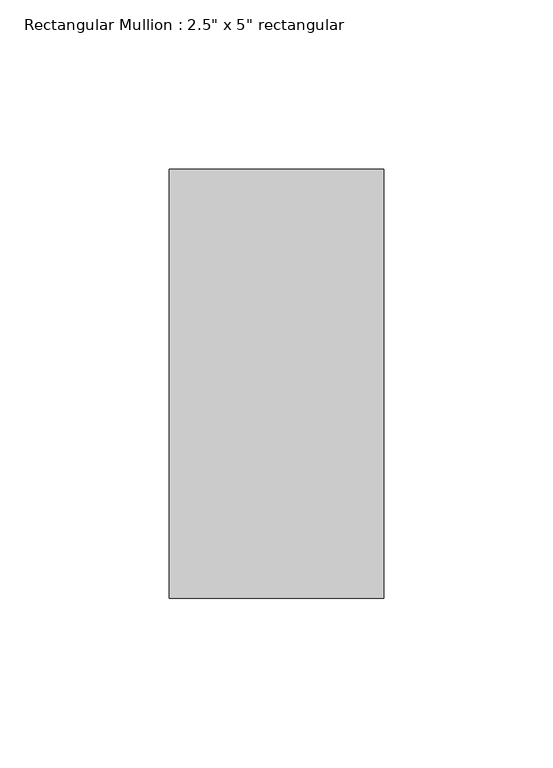
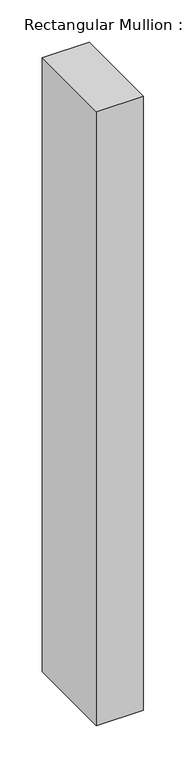
"""IFC4 building model written with IfcOpenShell, lengths in millimetres: member geometry."""

from ifc_helpers import new_model, si_unit, frame, origin, place, context, project, spatial, polyline, outline, extrude, source, transform, mapped, element, save


def member_5cd4c5ac(model_context):
    return source(origin(), model_context, "Body", "SweptSolid", [
        extrude(outline(polyline([(0.0, 63.5), (0.0, -63.5), (-63.5, -63.5), (-63.5, 63.5), (0.0, 63.5)])), frame((0.0, 0.0, -882.65), z_axis=(0.0, 0.0, 1.0), x_axis=(1.0, 0.0, 0.0)), (0.0, 0.0, 1.0), 882.65),
    ])


if __name__ == "__main__":
    model = new_model("IFC4")
    model_context = context("Model", 3, world=origin())
    ifc_project = project(units=[si_unit("LENGTHUNIT", "METRE", prefix="MILLI")], contexts=[model_context])
    site = spatial("IfcSite", under=ifc_project)
    building = spatial("IfcBuilding", under=site)
    placement = place(None, origin())
    member_shape = member_5cd4c5ac(model_context)
    element("IfcMember", 1, ObjectType="Rectangular Mullion : 2.5\" x 5\" rectangular", at=placement, inside=building, context=model_context, shape_type="MappedRepresentation", body=[
        mapped(member_shape, transform((0.0, 0.0, 0.0), x_axis=(1.0, 0.0, 0.0), y_axis=(0.0, 1.0, 0.0), z_axis=(0.0, 0.0, 1.0))),
    ])
    save(model, "model.ifc")

# Revit data of these elements
# Type "Rectangular Mullion : 2.5\" x 5\" rectangular"
#   built-in parameter 1007304 = 0.416667 (stored number, unit not read)
#   built-in parameter 1007301 = 0.104167 (stored number, unit not read)
#   built-in parameter 1007300 = 0.104167 (stored number, unit not read)
